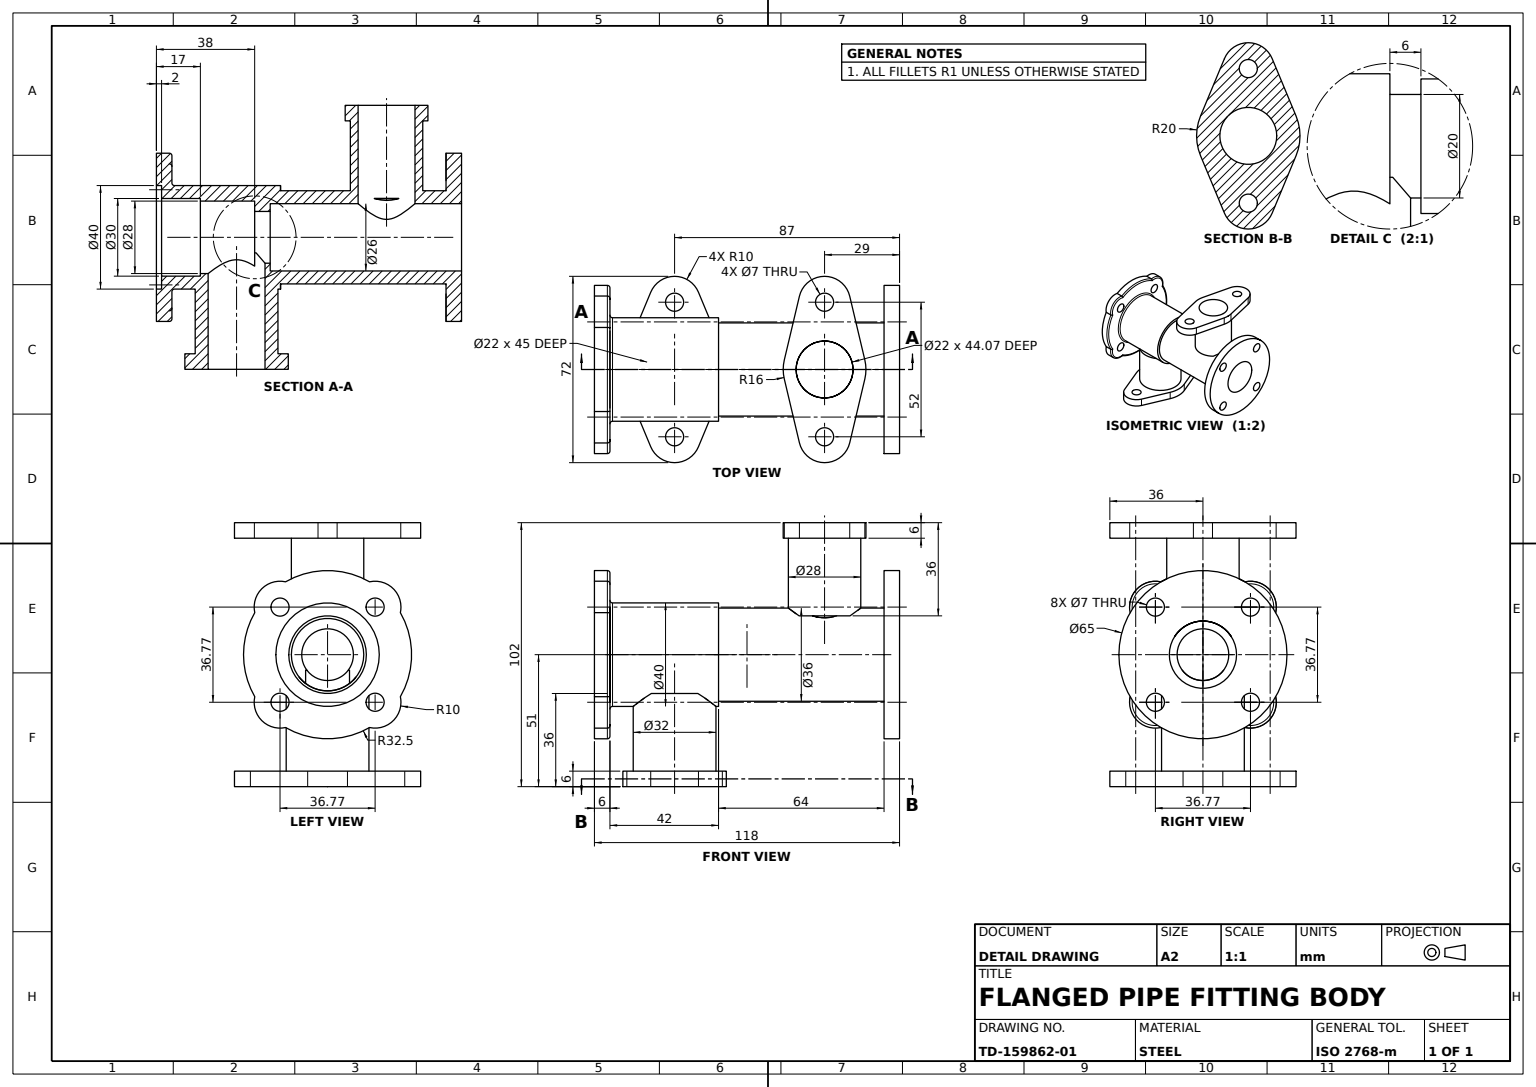
SolidWorks part; units mm, degrees
material "Plain Carbon Steel"
ref_plane "Front Plane" through (0, 0, 0) normal (0, 0, 1) x (1, 0, 0)
ref_plane "Top Plane" through (0, 0, 0) normal (0, 1, 0) x (1, 0, 0)
ref_plane "Right Plane" through (0, 0, 0) normal (1, 0, 0) x (0, 0, -1)
sketch "Bottom Flange Sketch" plane through (0, 0, 0) normal (0, 0, 1) x (1, 0, 0)
  circle A1 centre (0, 0) radius 32.5
  dimension "D1" = 65
extrude "Bottom Flange Ø65" add sketch "Bottom Flange Sketch" along normal blind 6
sketch "Lower Tube Sketch" plane through (0, 0, 6) normal (0, 0, 1) x (1, 0, 0)
  circle A0 centre (0, 0) radius 18
  dimension "D1" = 36
extrude "Lower Tube Ø36" add sketch "Lower Tube Sketch" along normal blind 64
sketch "Upper Tube Sketch" plane through (0, 0, 70) normal (0, 0, 1) x (1, 0, 0)
  circle A0 centre (0, 0) radius 20
  dimension "D1" = 40
extrude "Upper Tube Ø40" add sketch "Upper Tube Sketch" along normal blind 42
sketch "Top Flange Sketch" plane through (0, 0, 112) normal (0, 0, 1) x (1, 0, 0)
  circle A0 centre (0, 0) radius 32.5
  dimension "D1" = 65
extrude "Top Flange Ø65" add sketch "Top Flange Sketch" along normal blind 6
sketch "Lobed Plate Sketch" plane through (0, 0, 118) normal (0, 0, 1) x (1, 0, 0)
  line L0 (0, 0) -> (0, 26) construction
  line L1 (0, 0) -> (0, -26) construction
  line L2 (0, 0) -> (26, 0) construction
  line L3 (0, 0) -> (-26, 0) construction
  line L4 (0, 0) -> (18.3848, 18.3848) construction
  circle A0 centre (0, 0) radius 26 construction
  circle A1 centre (18.3848, 18.3848) radius 2.5
  arc A2 (28.1519, 16.2394) -> (16.2394, 28.1519) centre (18.3848, 18.3848) ccw
  circle A3 centre (0, 0) radius 32.5
  arc A4 (16.2394, -28.1519) -> (28.1519, -16.2394) centre (18.3848, -18.3848) ccw
  arc A5 (-28.1519, -16.2394) -> (-16.2394, -28.1519) centre (-18.3848, -18.3848) ccw
  arc A6 (-16.2394, 28.1519) -> (-28.1519, 16.2394) centre (-18.3848, 18.3848) ccw
  circle A7 centre (18.3848, -18.3848) radius 2.5
  circle A8 centre (-18.3848, -18.3848) radius 2.5
  circle A9 centre (-18.3848, 18.3848) radius 2.5
  circle M8 centre (0, 0) radius 32.5
  dimension "D1" = 52
  dimension "D3" = 5
  dimension "D4" = 20
  dimension "D5" = 65
  dimension "D7" = 18.3848
  dimension "D10" = 18.3848
  dimension "D2" = 45
  dimension "D8" = 18.3848
  dimension "D11" = 18.3848
  dimension "D6" = 4
  dimension "D9" = 4
extrude "Top Lobed Plate" add sketch "Lobed Plate Sketch" against normal blind 6 contours A3 A6 | A2 M8 | A3 A4 | A3 A5 | A9 | A1 | A7 | A8
sketch "Top Flange Holes Sketch" plane through (0, 0, 118) normal (0, 0, 1) x (1, 0, 0)
  line L0 (0, 0) -> (26, 0) construction
  line L1 (0, 0) -> (18.3848, 18.3848) construction
  circle A0 centre (0, 0) radius 26 construction
  circle A1 centre (18.3848, 18.3848) radius 3.5
  circle A2 centre (18.3848, -18.3848) radius 3.5
  circle A3 centre (-18.3848, -18.3848) radius 3.5
  circle A4 centre (-18.3848, 18.3848) radius 3.5
  dimension "D1" = 52
  dimension "D3" = 7
  dimension "D5" = 18.3848
  dimension "D2" = 45
  dimension "D6" = 18.3848
  dimension "D4" = 4
extrude "Top Flange Holes 4xØ7" cut sketch "Top Flange Holes Sketch" against normal blind 6
sketch "Bottom Flange Holes Sketch" plane through (0, 0, 0) normal (0, 0, -1) x (-1, 0, 0)
  line L0 (0, 0) -> (0, 26) construction
  line L1 (0, 0) -> (18.3848, 18.3848) construction
  circle A0 centre (0, 0) radius 26 construction
  circle A1 centre (18.3848, 18.3848) radius 3.5
  circle A2 centre (18.3848, -18.3848) radius 3.5
  circle A3 centre (-18.3848, -18.3848) radius 3.5
  circle A4 centre (-18.3848, 18.3848) radius 3.5
  dimension "D1" = 52
  dimension "D3" = 7
  dimension "D2" = 45
  dimension "D5" = 18.3848
  dimension "D6" = 18.3848
  dimension "D4" = 4
extrude "Bottom Flange Holes 4xØ7" cut sketch "Bottom Flange Holes Sketch" against normal blind 6
sketch "Top Counterbore Sketch" plane through (0, 0, 118) normal (0, 0, 1) x (1, 0, 0)
  circle A0 centre (0, 0) radius 20
  dimension "D1" = 40
extrude "Top Counterbore Ø40" cut sketch "Top Counterbore Sketch" against normal blind 2
sketch "Bore Ø30 Sketch" plane through (0, 0, 116) normal (0, 0, 1) x (1, 0, 0)
  circle A0 centre (0, 0) radius 15
  dimension "D1" = 30
extrude "Bore Ø30" cut sketch "Bore Ø30 Sketch" against normal blind 15
sketch "Bore Ø28 Sketch" plane through (0, 0, 101) normal (0, 0, 1) x (1, 0, 0)
  circle A0 centre (0, 0) radius 14
  dimension "D1" = 28
extrude "Bore Ø28" cut sketch "Bore Ø28 Sketch" against normal blind 21
sketch "Bore Ø20 Sketch" plane through (0, 0, 80) normal (0, 0, 1) x (1, 0, 0)
  circle A0 centre (0, 0) radius 10
  dimension "D1" = 20
extrude "Bore Ø20" cut sketch "Bore Ø20 Sketch" against normal blind 6
sketch "Bore Ø26 Sketch" plane through (0, 0, 74) normal (0, 0, 1) x (1, 0, 0)
  circle A0 centre (0, 0) radius 13
  dimension "D1" = 26
extrude "Bore Ø26" cut sketch "Bore Ø26 Sketch" against normal through all
ref_plane "Side Port 1 Plane" through (0, -15, 0) normal (0, 1, 0) x (1, 0, 0)
sketch "Side Port 1 Boss Sketch" plane through (0, -15, 0) normal (0, 1, 0) x (1, 0, 0)
  line L0 (0, 0) -> (0, -87) construction
  circle A0 centre (0, -87) radius 16
  dimension "D1" = 32
  dimension "D2" = 87
extrude "Side Port 1 Boss Ø32" add sketch "Side Port 1 Boss Sketch" against normal blind 30
sketch "Side Port 1 Flange Sketch" plane through (0, -45, 0) normal (0, -1, 0) x (1, 0, 0)
  line L0 (0, 87) -> (-26, 87) construction
  line L1 (0, 87) -> (26, 87) construction
  line L2 (-29.8462, 96.2308) -> (-7.6923, 105.4615)
  line L3 (7.6923, 105.4615) -> (29.8462, 96.2308)
  line L4 (-29.8462, 77.7692) -> (-7.6923, 68.5385)
  line L5 (7.6923, 68.5385) -> (29.8462, 77.7692)
  arc A0 (-7.6923, 68.5385) -> (7.6923, 68.5385) centre (0, 87) ccw
  arc A1 (-29.8462, 96.2308) -> (-29.8462, 77.7692) centre (-26, 87) ccw
  arc A2 (29.8462, 77.7692) -> (29.8462, 96.2308) centre (26, 87) ccw
  arc A3 (7.6923, 105.4615) -> (-7.6923, 105.4615) centre (0, 87) ccw
  dimension "D1" = 40
  dimension "D2" = 20
  dimension "D3" = 20
  dimension "D4" = 26
  dimension "D5" = 26
extrude "Side Port 1 Flange" add sketch "Side Port 1 Flange Sketch" along normal blind 6
sketch "Side Port 1 Holes Sketch" plane through (0, -51, 0) normal (0, -1, 0) x (1, 0, 0)
  circle A0 centre (-26, 87) radius 3.5
  circle A1 centre (26, 87) radius 3.5
  dimension "D1" = 7
  dimension "D2" = 7
extrude "Side Port 1 Holes 2xØ7" cut sketch "Side Port 1 Holes Sketch" against normal blind 6
fillet "Top Flange Fillet R1" radius 1 1 edges at (20, 0, 112)
fillet "Lobed Plate Fillet R1" radius 1 8 edges at (-25.4558, -25.4558, 112) (-32.5, 0, 112) (-25.4558, 25.4558, 112) (0, 32.5, 112) (25.4558, 25.4558, 112) (32.5, 0, 112) (25.4558, -25.4558, 112) (0, -32.5, 112)
sketch "Side Port 1 Bore Sketch" plane through (0, -51, 0) normal (0, -1, 0) x (1, 0, 0)
  circle A0 centre (0, 87) radius 11
  dimension "D1" = 22
extrude "Side Port 1 Bore Ø22" cut sketch "Side Port 1 Bore Sketch" against normal blind 45
ref_plane "Side Port 2 Plane" through (0, 15, 0) normal (0, 1, 0) x (1, 0, 0)
sketch "Side Port 2 Boss Sketch" plane through (0, 15, 0) normal (0, 1, 0) x (1, 0, 0)
  line L0 (0, 0) -> (0, -29) construction
  circle A0 centre (0, -29) radius 14
  dimension "D1" = 28
  dimension "D2" = 29
extrude "Side Port 2 Boss Ø28" add sketch "Side Port 2 Boss Sketch" along normal blind 30
sketch "Side Port 2 Flange Sketch" plane through (0, 45, 0) normal (0, 1, 0) x (1, 0, 0)
  line L0 (0, -29) -> (-26, -29) construction
  line L1 (0, -29) -> (26, -29) construction
  line L2 (-28.3077, -19.2699) -> (-3.6923, -13.4319)
  line L3 (3.6923, -13.4319) -> (28.3077, -19.2699)
  line L4 (-28.3077, -38.7301) -> (-3.6923, -44.5681)
  line L5 (3.6923, -44.5681) -> (28.3077, -38.7301)
  arc A0 (-3.6923, -44.5681) -> (3.6923, -44.5681) centre (0, -29) ccw
  arc A1 (-28.3077, -19.2699) -> (-28.3077, -38.7301) centre (-26, -29) ccw
  arc A2 (28.3077, -38.7301) -> (28.3077, -19.2699) centre (26, -29) ccw
  arc A3 (3.6923, -13.4319) -> (-3.6923, -13.4319) centre (0, -29) ccw
  dimension "D1" = 32
  dimension "D2" = 20
  dimension "D3" = 20
  dimension "D4" = 26
  dimension "D5" = 26
extrude "Side Port 2 Flange" add sketch "Side Port 2 Flange Sketch" along normal blind 6
sketch "Side Port 2 Holes Sketch" plane through (0, 51, 0) normal (0, 1, 0) x (1, 0, 0)
  circle A0 centre (-26, -29) radius 3.5
  circle A1 centre (26, -29) radius 3.5
  dimension "D1" = 7
  dimension "D2" = 7
extrude "Side Port 2 Holes 2xØ7" cut sketch "Side Port 2 Holes Sketch" against normal blind 6
sketch "Side Port 2 Bore Sketch" plane through (0, 51, 0) normal (0, 1, 0) x (1, 0, 0)
  circle A0 centre (0, -29) radius 11
  dimension "D1" = 22
extrude "Side Port 2 Bore Ø22" cut sketch "Side Port 2 Bore Sketch" against normal blind 45
